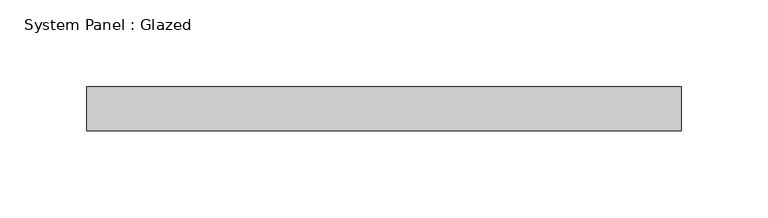
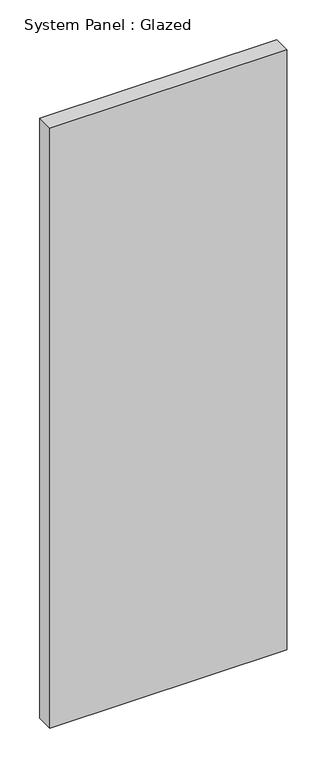
"""IFC4 building model written with IfcOpenShell, lengths in millimetres: plate geometry, System Panel : Glazed."""

from ifc_helpers import new_model, si_unit, origin, origin_with_axes, place, context, project, spatial, polyline, outline, extrude, source, transform, mapped, element, save


def system_panel_glazed_b83167b9(model_context):
    return source(origin(), model_context, "Body", "SweptSolid", [
        extrude(outline(polyline([(171.45, 19.05), (-171.45, 19.05), (-171.45, 44.45), (171.45, 44.45), (171.45, 19.05)])), origin_with_axes(), (0.0, 0.0, 1.0), 918.6333333),
    ])


if __name__ == "__main__":
    model = new_model("IFC4")
    model_context = context("Model", 3, world=origin())
    ifc_project = project(units=[si_unit("LENGTHUNIT", "METRE", prefix="MILLI")], contexts=[model_context])
    site = spatial("IfcSite", under=ifc_project)
    building = spatial("IfcBuilding", under=site)
    placement = place(None, origin())
    system_panel_glazed_shape = system_panel_glazed_b83167b9(model_context)
    element("IfcPlate", 1, ObjectType="System Panel : Glazed", at=placement, inside=building, context=model_context, shape_type="MappedRepresentation", body=[
        mapped(system_panel_glazed_shape, transform((0.0, 0.0, 0.0), x_axis=(1.0, 0.0, 0.0), y_axis=(0.0, 1.0, 0.0), z_axis=(0.0, 0.0, 1.0))),
    ])
    save(model, "model.ifc")

# Revit data of these elements
# Type "System Panel : Glazed"
#   Construction Type Id = "GSP4R"
#   Analytic Construction = "1/8 in Pilkington single glazing"
#   Visual Light Transmittance = 0.9
#   Solar Heat Gain Coefficient = 0.86
#   Heat Transfer Coefficient (U) = 1.18115 BTU/(h·ft²·°F)
# Element 1 (IfcPlate, "System Panel : Glazed")
#   Materials on its faces: "Glass"
# Materials
#   "Glass": class "Glass", colour RGB 0 128 192, transparency 0.75, Description = "Soda Lime Glass", Cost = 0
